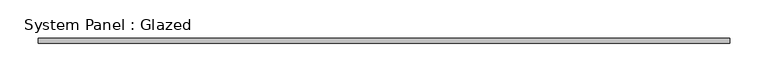
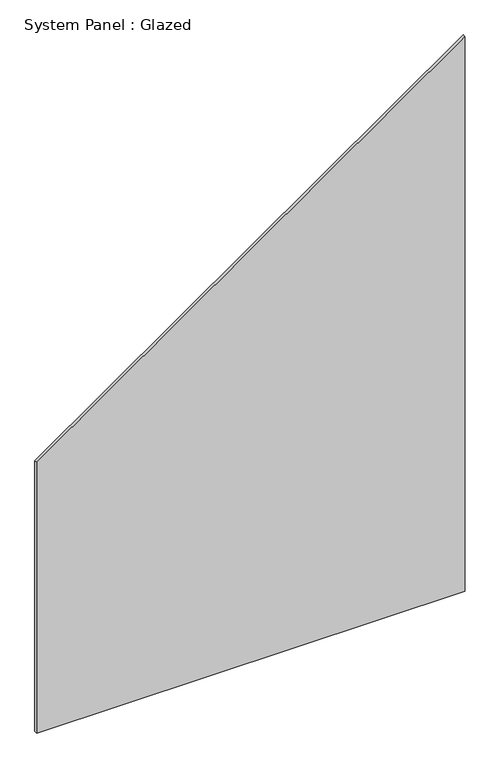
"""IFC4 building model written with IfcOpenShell, lengths in millimetres: plate geometry, System Panel : Glazed."""

from ifc_helpers import new_model, si_unit, frame, origin, place, context, project, spatial, polyline, outline, extrude, source, transform, mapped, element, save


def system_panel_glazed_94ea2f12(model_context):
    return source(origin(), model_context, "Body", "SweptSolid", [
        extrude(outline(polyline([(0.0, -450.0), (0.0, 450.0), (1230.8328815, 450.0), (600.6460971, -450.0), (0.0, -450.0)])), frame((0.0, 34.0, 0.0), z_axis=(0.0, 1.0, 0.0), x_axis=(0.0, 0.0, 1.0)), (0.0, 0.0, 1.0), 6.0),
    ])


if __name__ == "__main__":
    model = new_model("IFC4")
    model_context = context("Model", 3, world=origin())
    ifc_project = project(units=[si_unit("LENGTHUNIT", "METRE", prefix="MILLI")], contexts=[model_context])
    site = spatial("IfcSite", under=ifc_project)
    building = spatial("IfcBuilding", under=site)
    placement = place(None, origin())
    system_panel_glazed_shape = system_panel_glazed_94ea2f12(model_context)
    element("IfcPlate", 1, ObjectType="System Panel : Glazed", at=placement, inside=building, context=model_context, shape_type="MappedRepresentation", body=[
        mapped(system_panel_glazed_shape, transform((0.0, 0.0, 0.0), x_axis=(1.0, 0.0, 0.0), y_axis=(0.0, 1.0, 0.0), z_axis=(0.0, 0.0, 1.0))),
    ])
    save(model, "model.ifc")

# Revit data of these elements
# Type "System Panel : Glazed"
#   Construction Type Id = "GSP4R"
#   Analytic Construction = "1/8 in Pilkington single glazing"
#   Visual Light Transmittance = 0.9
#   Solar Heat Gain Coefficient = 0.86
#   Heat Transfer Coefficient (U) = 6.7069 W/(m²·K)
#   Define Thermal Properties by = 1
# Element 1 (IfcPlate, "System Panel : Glazed")
#   Materials on its faces: "Default New Material(6)"
# Materials
#   "Default New Material(6)": class "Generic", colour RGB 191 25 25, transparency 0.9, Cost = 0
